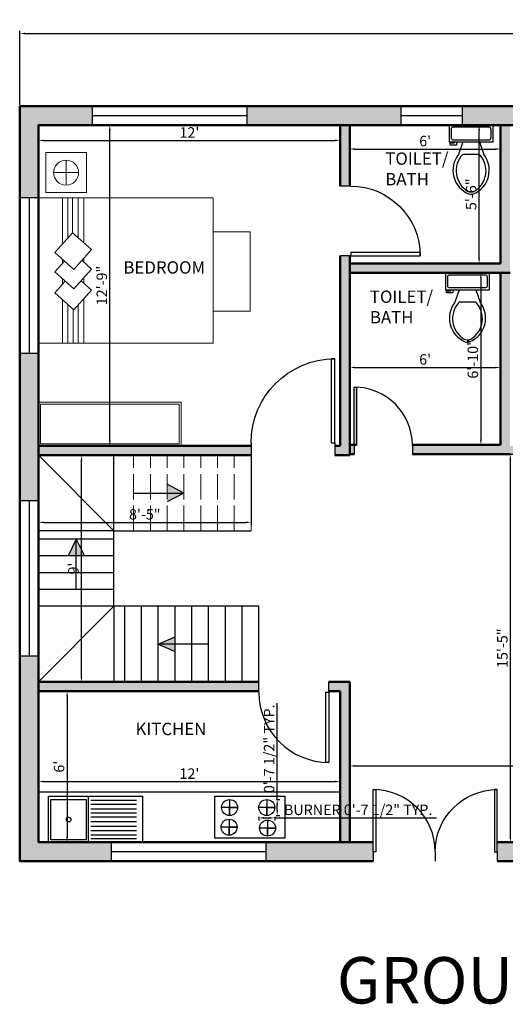
# Model space of a CAD drawing. Units: inches. Extents: x 1882 to 2467, y 1298 to 1767.
# Tile 1 of 2: x 1882 to 2114, y 1298 to 1767. Entities that reach past the tile are written whole.
import ezdxf

# ---------------------------------------------------------------- set-up
doc = ezdxf.new("R2010")
doc.units = ezdxf.units.IN
doc.linetypes.add('ACAD_ISO02W100', pattern=[15, 12, -3])
for name, color, linetype, lineweight in [('A-ANNO-DIMS', 2, 'Continuous', 18), ('A-ANNO-TEXT', 7, 'Continuous', 35), ('A-AREA-IDEN', 7, 'Continuous', 25), ('A-FLOR-FIXT', 9, 'Continuous', 25), ('A-FLOR-STRS', 7, 'Continuous', 25), ('A-FLOR-STRS-OVHD', 7, 'ACAD_ISO02W100', 18), ('A-FLOR-STRS-PATT', 7, 'Continuous', 13), ('A-FURN', 8, 'Continuous', 18), ('A-WALL-PATT', 160, 'Continuous', 13), ('DOOR', 140, 'Continuous', 25), ('KIT', 10, 'Continuous', 25), ('WALL', 160, 'Continuous', 50), ('WIND', 52, 'Continuous', 25)]:
    doc.layers.add(name, color=color, linetype=linetype, lineweight=lineweight)
doc.styles.get("Standard").update_dxf_attribs({"font": 'arial.ttf'})
doc.dimstyles.new('ISO-25', dxfattribs={"dimtxt": 5, "dimasz": 2.5, "dimexe": 1.25, "dimexo": 0.625, "dimtad": 1, "dimdec": 0, "dimlunit": 4, "dimtxsty": 'Standard', "dimcen": 2.5, "dimadec": 0, "dimazin": 0, "dimtfac": 1, "dimtdec": 0, "dimtmove": 0, "dimatfit": 3, "dimfxl": 1, "dimarcsym": 0})

# ---------------------------------------------------------------- blocks, each defined once
blk = doc.blocks.new('*U2')
for p, q in [((0, 0), (0, -6)), ((40, 0), (40, -6))]:
    blk.add_line(p, q)
blk.add_lwpolyline([(0, 0), (0, 40), (1.75, 40), (1.75, 0)], close=True)
blk.add_arc((0, 0), 40, 0, 90)
blk = doc.blocks.new('*U4')
for p, q in [((9.5, -6), (9.5, -2)), ((-10, -8.5), (-8, -8.5)), ((-10, -9.5), (-10, -8.5)), ((-8, -8.5), (-8, -8)), ((-7, -8), (-7, -9.5)), ((-4, -8), (-6, -14)), ((4, -8), (6, -14)), ((-7, -9.5), (-10, -9.5)), ((4, -14), (-4, -14))]:
    blk.add_line(p, q)
blk.add_lwpolyline([(10.5, -8), (10.5, 0), (-10.5, 0), (-10.5, -8)], close=True)
for points in [[(-9.5, -2), (-9.5, -6)], [(8.5, -1), (-8.5, -1)], [(-8.5, -7), (8.5, -7)]]:
    blk.add_lwpolyline(points)
for centre, radius, start, end in [((-8.62, -1.88), 0.884, 81.8699, 188.1301), ((8.62, -1.88), 0.884, 351.8699, 98.1301), ((-8.62, -6.12), 0.884, 171.8699, 278.1301), ((8.62, -6.12), 0.884, 261.8699, 8.1301), ((3.52, -21.58), 12.17, 141.4691, 247.9714), ((4.2, -21.82), 11.33, 136.3677, 238.9468), ((-3.52, -21.58), 12.17, 292.0284, 38.5307), ((-4.2, -21.82), 11.33, 301.053, 43.6321), ((0, -27.88), 4, 245.7318, 294.2682), ((0, -29), 4, 254.8605, 285.1395)]:
    blk.add_arc(centre, radius, start, end)
blk = doc.blocks.new('*D7')
at = {"layer": 'A-ANNO-DIMS', "color": 0, "lineweight": -2, "transparency": 16777216}
for p, q in [((1891.22, 1716.45), (1891.22, 1708.51)), ((2035.22, 1716.45), (2035.22, 1708.51)), ((1893.72, 1709.76), (2032.72, 1709.76))]:
    blk.add_line(p, q, dxfattribs=at)
at = {"layer": 'A-ANNO-DIMS', "color": 0, "lineweight": 100, "transparency": 16777216}
for points in [[(1893.72, 1710.18), (1893.72, 1709.35), (1891.22, 1709.76)], [(2032.72, 1710.18), (2032.72, 1709.35), (2035.22, 1709.76)]]:
    blk.add_solid(points, dxfattribs=at)
at = {"layer": 'Defpoints', "color": 0, "lineweight": 100, "transparency": 16777216}
for p in [(1891.22, 1717.07), (2035.22, 1717.07), (2035.22, 1709.76)]:
    blk.add_point(p, dxfattribs=at)
at = {"layer": 'A-ANNO-DIMS', "color": 0, "transparency": 16777216, "insert": (1963.22, 1712.9), "char_height": 5, "attachment_point": 5}
blk.add_mtext("12'", dxfattribs=at)
blk = doc.blocks.new('*D8')
at = {"layer": 'A-ANNO-DIMS', "color": 0, "lineweight": -2, "transparency": 16777216}
for p, q in [((1891.84, 1717.07), (1926.48, 1717.07)), ((1925.23, 1566.57), (1925.23, 1714.57)), ((1891.84, 1564.07), (1926.48, 1564.07))]:
    blk.add_line(p, q, dxfattribs=at)
at = {"layer": 'A-ANNO-DIMS', "color": 0, "lineweight": 100, "transparency": 16777216}
for points in [[(1924.81, 1714.57), (1925.64, 1714.57), (1925.23, 1717.07)], [(1924.81, 1566.57), (1925.64, 1566.57), (1925.23, 1564.07)]]:
    blk.add_solid(points, dxfattribs=at)
at = {"layer": 'Defpoints', "color": 0, "lineweight": 100, "transparency": 16777216}
for p in [(1891.22, 1717.07), (1925.23, 1717.07), (1891.22, 1564.07)]:
    blk.add_point(p, dxfattribs=at)
at = {"layer": 'A-ANNO-DIMS', "color": 0, "transparency": 16777216, "insert": (1922.05, 1640.57), "char_height": 5, "attachment_point": 5, "rotation": 90}
blk.add_mtext('12\'-9"', dxfattribs=at)
blk = doc.blocks.new('*D9')
at = {"layer": 'A-ANNO-DIMS', "color": 0, "lineweight": -2, "transparency": 16777216}
for p, q in [((2039.72, 1716.45), (2039.72, 1704.39)), ((2111.72, 1716.45), (2111.72, 1704.39)), ((2042.22, 1705.64), (2109.22, 1705.64))]:
    blk.add_line(p, q, dxfattribs=at)
at = {"layer": 'A-ANNO-DIMS', "color": 0, "lineweight": 100, "transparency": 16777216}
for points in [[(2042.22, 1706.05), (2042.22, 1705.22), (2039.72, 1705.64)], [(2109.22, 1706.05), (2109.22, 1705.22), (2111.72, 1705.64)]]:
    blk.add_solid(points, dxfattribs=at)
at = {"layer": 'Defpoints', "color": 0, "lineweight": 100, "transparency": 16777216}
for p in [(2039.72, 1717.07), (2111.72, 1717.07), (2111.72, 1705.64)]:
    blk.add_point(p, dxfattribs=at)
at = {"layer": 'A-ANNO-DIMS', "color": 0, "transparency": 16777216, "insert": (2075.72, 1708.81), "char_height": 5, "attachment_point": 5}
blk.add_mtext("6'", dxfattribs=at)
blk = doc.blocks.new('*D10')
at = {"layer": 'A-ANNO-DIMS', "color": 0, "lineweight": -2, "transparency": 16777216}
for p, q in [((2111.09, 1717.07), (2100.22, 1717.07)), ((2101.47, 1653.57), (2101.47, 1714.57)), ((2111.09, 1651.07), (2100.22, 1651.07))]:
    blk.add_line(p, q, dxfattribs=at)
at = {"layer": 'A-ANNO-DIMS', "color": 0, "lineweight": 100, "transparency": 16777216}
for points in [[(2101.05, 1714.57), (2101.89, 1714.57), (2101.47, 1717.07)], [(2101.05, 1653.57), (2101.89, 1653.57), (2101.47, 1651.07)]]:
    blk.add_solid(points, dxfattribs=at)
at = {"layer": 'Defpoints', "color": 0, "lineweight": 100, "transparency": 16777216}
for p in [(2101.47, 1717.07), (2111.72, 1717.07), (2111.72, 1651.07)]:
    blk.add_point(p, dxfattribs=at)
at = {"layer": 'A-ANNO-DIMS', "color": 0, "transparency": 16777216, "insert": (2098.29, 1684.07), "char_height": 5, "attachment_point": 5, "rotation": 90}
blk.add_mtext('5\'-6"', dxfattribs=at)
blk = doc.blocks.new('*D17')
at = {"layer": 'A-ANNO-DIMS', "color": 0, "lineweight": -2, "transparency": 16777216}
for p, q in [((2039.72, 1375.7), (2039.72, 1412.69)), ((2042.22, 1411.44), (2336.72, 1411.44)), ((2339.22, 1375.7), (2339.22, 1412.69))]:
    blk.add_line(p, q, dxfattribs=at)
at = {"layer": 'A-ANNO-DIMS', "color": 0, "lineweight": 100, "transparency": 16777216}
for points in [[(2042.22, 1411.86), (2042.22, 1411.02), (2039.72, 1411.44)], [(2336.72, 1411.86), (2336.72, 1411.02), (2339.22, 1411.44)]]:
    blk.add_solid(points, dxfattribs=at)
at = {"layer": 'Defpoints', "color": 0, "lineweight": 100, "transparency": 16777216}
for p in [(2339.22, 1411.44), (2039.72, 1375.07), (2339.22, 1375.07)]:
    blk.add_point(p, dxfattribs=at)
at = {"layer": 'A-ANNO-DIMS', "color": 0, "transparency": 16777216, "insert": (2189.47, 1414.62), "char_height": 5, "attachment_point": 5}
blk.add_mtext("25'", dxfattribs=at)
blk = doc.blocks.new('*D18')
at = {"layer": 'A-ANNO-DIMS', "color": 0, "lineweight": -2, "transparency": 16777216}
for p, q in [((1891.22, 1375.7), (1891.22, 1405.24)), ((2035.22, 1375.7), (2035.22, 1405.24)), ((1893.72, 1403.99), (2032.72, 1403.99))]:
    blk.add_line(p, q, dxfattribs=at)
at = {"layer": 'A-ANNO-DIMS', "color": 0, "lineweight": 100, "transparency": 16777216}
for points in [[(1893.72, 1404.4), (1893.72, 1403.57), (1891.22, 1403.99)], [(2032.72, 1404.4), (2032.72, 1403.57), (2035.22, 1403.99)]]:
    blk.add_solid(points, dxfattribs=at)
at = {"layer": 'Defpoints', "color": 0, "lineweight": 100, "transparency": 16777216}
for p in [(2035.22, 1403.99), (1891.22, 1375.07), (2035.22, 1375.07)]:
    blk.add_point(p, dxfattribs=at)
at = {"layer": 'A-ANNO-DIMS', "color": 0, "transparency": 16777216, "insert": (1963.22, 1407.12), "char_height": 5, "attachment_point": 5}
blk.add_mtext("12'", dxfattribs=at)
blk = doc.blocks.new('*D19')
at = {"layer": 'A-ANNO-DIMS', "color": 0, "lineweight": -2, "transparency": 16777216}
for p, q in [((1891.84, 1447.07), (1906.1, 1447.07)), ((1904.85, 1444.57), (1904.85, 1377.57)), ((1891.84, 1375.07), (1906.1, 1375.07))]:
    blk.add_line(p, q, dxfattribs=at)
at = {"layer": 'A-ANNO-DIMS', "color": 0, "lineweight": 100, "transparency": 16777216}
for points in [[(1904.43, 1444.57), (1905.27, 1444.57), (1904.85, 1447.07)], [(1904.43, 1377.57), (1905.27, 1377.57), (1904.85, 1375.07)]]:
    blk.add_solid(points, dxfattribs=at)
at = {"layer": 'Defpoints', "color": 0, "lineweight": 100, "transparency": 16777216}
for p in [(1891.22, 1447.07), (1891.22, 1375.07), (1904.85, 1375.07)]:
    blk.add_point(p, dxfattribs=at)
at = {"layer": 'A-ANNO-DIMS', "color": 0, "transparency": 16777216, "insert": (1901.67, 1411.07), "char_height": 5, "attachment_point": 5, "rotation": 90}
blk.add_mtext("6'", dxfattribs=at)
blk = doc.blocks.new('*D20')
at = {"layer": 'A-ANNO-DIMS', "color": 0, "lineweight": -2, "transparency": 16777216}
for p, q in [((1891.84, 1559.57), (1912.93, 1559.57)), ((1911.68, 1454.07), (1911.68, 1557.07)), ((1891.84, 1451.57), (1912.93, 1451.57))]:
    blk.add_line(p, q, dxfattribs=at)
at = {"layer": 'A-ANNO-DIMS', "color": 0, "lineweight": 100, "transparency": 16777216}
for points in [[(1911.27, 1557.07), (1912.1, 1557.07), (1911.68, 1559.57)], [(1911.27, 1454.07), (1912.1, 1454.07), (1911.68, 1451.57)]]:
    blk.add_solid(points, dxfattribs=at)
at = {"layer": 'Defpoints', "color": 0, "lineweight": 100, "transparency": 16777216}
for p in [(1891.22, 1559.57), (1911.68, 1559.57), (1891.22, 1451.57)]:
    blk.add_point(p, dxfattribs=at)
at = {"layer": 'A-ANNO-DIMS', "color": 0, "transparency": 16777216, "insert": (1908.51, 1505.57), "char_height": 5, "attachment_point": 5, "rotation": 90}
blk.add_mtext("9'", dxfattribs=at)
blk = doc.blocks.new('*D21')
at = {"layer": 'A-ANNO-DIMS', "color": 0, "lineweight": -2, "transparency": 16777216}
for p, q in [((1891.22, 1558.95), (1891.22, 1526.34)), ((1992.61, 1558.95), (1992.61, 1526.34)), ((1893.72, 1527.59), (1990.11, 1527.59))]:
    blk.add_line(p, q, dxfattribs=at)
at = {"layer": 'A-ANNO-DIMS', "color": 0, "lineweight": 100, "transparency": 16777216}
for points in [[(1893.72, 1528.01), (1893.72, 1527.17), (1891.22, 1527.59)], [(1990.11, 1528.01), (1990.11, 1527.17), (1992.61, 1527.59)]]:
    blk.add_solid(points, dxfattribs=at)
at = {"layer": 'Defpoints', "color": 0, "lineweight": 100, "transparency": 16777216}
for p in [(1891.22, 1559.57), (1992.61, 1559.57), (1992.61, 1527.59)]:
    blk.add_point(p, dxfattribs=at)
at = {"layer": 'A-ANNO-DIMS', "color": 0, "transparency": 16777216, "insert": (1941.92, 1530.77), "char_height": 5, "attachment_point": 5}
blk.add_mtext('8\'-5"', dxfattribs=at)
blk = doc.blocks.new('*D22')
at = {"layer": 'A-ANNO-DIMS', "color": 0, "lineweight": -2, "transparency": 16777216}
for p, q in [((2039.72, 1645.95), (2039.72, 1600.23)), ((2111.72, 1645.95), (2111.72, 1600.23)), ((2042.22, 1601.48), (2109.22, 1601.48))]:
    blk.add_line(p, q, dxfattribs=at)
at = {"layer": 'A-ANNO-DIMS', "color": 0, "lineweight": 100, "transparency": 16777216}
for points in [[(2042.22, 1601.89), (2042.22, 1601.06), (2039.72, 1601.48)], [(2109.22, 1601.89), (2109.22, 1601.06), (2111.72, 1601.48)]]:
    blk.add_solid(points, dxfattribs=at)
at = {"layer": 'Defpoints', "color": 0, "lineweight": 100, "transparency": 16777216}
for p in [(2039.72, 1646.57), (2111.72, 1646.57), (2111.72, 1601.48)]:
    blk.add_point(p, dxfattribs=at)
at = {"layer": 'A-ANNO-DIMS', "color": 0, "transparency": 16777216, "insert": (2075.72, 1604.65), "char_height": 5, "attachment_point": 5}
blk.add_mtext("6'", dxfattribs=at)
blk = doc.blocks.new('*D23')
at = {"layer": 'A-ANNO-DIMS', "color": 0, "lineweight": -2, "transparency": 16777216}
for p, q in [((2111.09, 1646.57), (2101.04, 1646.57)), ((2102.29, 1644.07), (2102.29, 1567.07)), ((2111.09, 1564.57), (2101.04, 1564.57))]:
    blk.add_line(p, q, dxfattribs=at)
at = {"layer": 'A-ANNO-DIMS', "color": 0, "lineweight": 100, "transparency": 16777216}
for points in [[(2101.87, 1644.07), (2102.7, 1644.07), (2102.29, 1646.57)], [(2101.87, 1567.07), (2102.7, 1567.07), (2102.29, 1564.57)]]:
    blk.add_solid(points, dxfattribs=at)
at = {"layer": 'Defpoints', "color": 0, "lineweight": 100, "transparency": 16777216}
for p in [(2111.72, 1646.57), (2102.29, 1564.57), (2111.72, 1564.57)]:
    blk.add_point(p, dxfattribs=at)
at = {"layer": 'A-ANNO-DIMS', "color": 0, "transparency": 16777216, "insert": (2099.11, 1605.57), "char_height": 5, "attachment_point": 5, "rotation": 90}
blk.add_mtext('6\'-10"', dxfattribs=at)
blk = doc.blocks.new('*D24')
at = {"layer": 'A-ANNO-DIMS', "color": 0, "lineweight": -2, "transparency": 16777216}
for p, q in [((2110.74, 1560.07), (2117.62, 1560.07)), ((2116.37, 1377.57), (2116.37, 1557.57)), ((2110.74, 1375.07), (2117.62, 1375.07))]:
    blk.add_line(p, q, dxfattribs=at)
at = {"layer": 'A-ANNO-DIMS', "color": 0, "lineweight": 100, "transparency": 16777216}
for points in [[(2115.96, 1557.57), (2116.79, 1557.57), (2116.37, 1560.07)], [(2115.96, 1377.57), (2116.79, 1377.57), (2116.37, 1375.07)]]:
    blk.add_solid(points, dxfattribs=at)
at = {"layer": 'Defpoints', "color": 0, "lineweight": 100, "transparency": 16777216}
for p in [(2110.11, 1560.07), (2116.37, 1560.07), (2110.11, 1375.07)]:
    blk.add_point(p, dxfattribs=at)
at = {"layer": 'A-ANNO-DIMS', "color": 0, "transparency": 16777216, "insert": (2113.2, 1467.57), "char_height": 5, "attachment_point": 5, "rotation": 90}
blk.add_mtext('15\'-5"', dxfattribs=at)
blk = doc.blocks.new('*D26')
at = {"layer": 'A-ANNO-DIMS', "color": 0, "lineweight": -2, "transparency": 16777216}
for p, q in [((1882.22, 1726.7), (1882.22, 1762.02)), ((2422.22, 1726.7), (2422.22, 1762.02)), ((1884.72, 1760.77), (2419.72, 1760.77))]:
    blk.add_line(p, q, dxfattribs=at)
at = {"layer": 'A-ANNO-DIMS', "color": 0, "lineweight": 100, "transparency": 16777216}
for points in [[(1884.72, 1761.18), (1884.72, 1760.35), (1882.22, 1760.77)], [(2419.72, 1761.18), (2419.72, 1760.35), (2422.22, 1760.77)]]:
    blk.add_solid(points, dxfattribs=at)
at = {"layer": 'Defpoints', "color": 0, "lineweight": 100, "transparency": 16777216}
for p in [(2422.22, 1760.77), (1882.22, 1726.07), (2422.22, 1726.07)]:
    blk.add_point(p, dxfattribs=at)
at = {"layer": 'A-ANNO-DIMS', "color": 0, "transparency": 16777216, "insert": (2152.22, 1763.93), "char_height": 5, "attachment_point": 5}
blk.add_mtext("45'", dxfattribs=at)
blk = doc.blocks.new('WIN-74IN')
blk.add_line((0, 4.5), (74.03, 4.5))
blk.add_lwpolyline([(0, 0), (74.03, 0), (74.03, 9), (0, 9)], close=True)
blk = doc.blocks.new('BED-DOUBLE')
for p, q in [((11.49, 47.34), (11.49, 69.21)), ((14, 50.17), (14, 69.21)), ((16.17, 52.63), (16.17, 69.21)), ((18.98, 50.15), (18.98, 69.21)), ((21.58, 47.84), (21.58, 69.21)), ((11.49, 38.12), (11.49, 39.83)), ((21.58, 38.62), (21.58, 40.3)), ((11.49, 28.1), (11.49, 30.61)), ((21.58, 28.61), (21.58, 31.07)), ((11.49, 0), (11.49, 20.59)), ((21.58, 0), (21.58, 21.06)), ((14, 0), (14, 18.37)), ((16.55, 0), (16.55, 16.12)), ((18.98, 0), (18.98, 18.12))]:
    blk.add_line(p, q)
for points in [[(0, 69.21), (83.41, 69.21), (83.41, 0), (0, 0)], [(7.76, 43.13), (16.17, 52.63), (25.33, 44.53), (16.92, 35.02)], [(83.41, 15.22), (100.98, 15.22), (100.98, 53.07), (83.41, 53.07)]]:
    blk.add_lwpolyline(points, close=True)
for points in [[(20.75, 39.36), (25.33, 35.3), (16.92, 25.8), (7.76, 33.9), (12.34, 39.08)], [(20.36, 29.69), (25.33, 25.29), (16.92, 15.79), (7.76, 23.89), (12.73, 29.51)]]:
    blk.add_lwpolyline(points)
blk = doc.blocks.new('NIGHTSTAND-LAMP')
for p, q in [((9.73, 9.55), (9.73, 15.52)), ((9.73, 15.52), (9.73, 3.59)), ((15.7, 9.55), (3.77, 9.55)), ((9.73, 3.59), (9.73, 9.55)), ((9.73, 9.55), (15.7, 9.55))]:
    blk.add_line(p, q)
blk.add_lwpolyline([(0, 0), (19.47, 0), (19.47, 19.1), (0, 19.1)], close=True)
blk.add_circle((9.73, 9.55), 5.97)
blk = doc.blocks.new('COOKTOP-BURNER')
for p, q in [((3.82, 7.64), (3.82, 0)), ((7.64, 3.82), (0, 3.82)), ((3.82, 0), (3.82, 3.82)), ((3.82, 3.82), (7.64, 3.82))]:
    blk.add_line(p, q)
blk.add_circle((3.82, 3.82), 3.82)
blk = doc.blocks.new('*D35')
at = {"layer": 'A-ANNO-DIMS', "color": 0, "lineweight": -2, "transparency": 16777216}
for p, q in [((1996.32, 1387.16), (1996.32, 1385.39)), ((1998.82, 1386.64), (2001.46, 1386.64)), ((2003.96, 1387.16), (2003.96, 1385.39)), ((2003.96, 1386.64), (2081.06, 1386.64))]:
    blk.add_line(p, q, dxfattribs=at)
at = {"layer": 'A-ANNO-DIMS', "color": 0, "lineweight": 100, "transparency": 16777216}
for points in [[(1998.82, 1387.05), (1998.82, 1386.22), (1996.32, 1386.64)], [(2001.46, 1387.05), (2001.46, 1386.22), (2003.96, 1386.64)]]:
    blk.add_solid(points, dxfattribs=at)
at = {"layer": 'Defpoints', "color": 0, "lineweight": 100, "transparency": 16777216}
for p in [(1996.32, 1387.78), (2003.96, 1387.78), (2003.96, 1386.64)]:
    blk.add_point(p, dxfattribs=at)
at = {"layer": 'A-ANNO-DIMS', "color": 0, "transparency": 16777216, "insert": (2043.76, 1389.85), "char_height": 5, "attachment_point": 5}
blk.add_mtext('BURNER 0\'-7 1/2" TYP.', dxfattribs=at)
blk = doc.blocks.new('*D36')
at = {"layer": 'A-ANNO-DIMS', "color": 0, "lineweight": -2, "transparency": 16777216}
for p, q in [((2005.11, 1395.42), (2005.11, 1441.3)), ((2004.59, 1395.42), (2006.36, 1395.42)), ((2005.11, 1390.28), (2005.11, 1392.92)), ((2004.59, 1387.78), (2006.36, 1387.78))]:
    blk.add_line(p, q, dxfattribs=at)
at = {"layer": 'A-ANNO-DIMS', "color": 0, "lineweight": 100, "transparency": 16777216}
for points in [[(2004.69, 1392.92), (2005.53, 1392.92), (2005.11, 1395.42)], [(2004.69, 1390.28), (2005.53, 1390.28), (2005.11, 1387.78)]]:
    blk.add_solid(points, dxfattribs=at)
at = {"layer": 'Defpoints', "color": 0, "lineweight": 100, "transparency": 16777216}
for p in [(2003.96, 1395.42), (2005.11, 1395.42), (2003.96, 1387.78)]:
    blk.add_point(p, dxfattribs=at)
at = {"layer": 'A-ANNO-DIMS', "color": 0, "transparency": 16777216, "insert": (2001.9, 1419.61), "char_height": 5, "attachment_point": 5, "rotation": 90}
blk.add_mtext('0\'-7 1/2" TYP.', dxfattribs=at)

msp = doc.modelspace()

# ---------------------------------------------------------------- hatches: boundary and pattern name
at = {"layer": 'A-FLOR-STRS-PATT'}
h = msp.add_hatch(color=256, dxfattribs=at)
h.dxf.hatch_style = 1
h.paths.add_polyline_path([(1960.61, 1541.57), (1952.61, 1541.57), (1952.61, 1537.32)])
h.paths.add_polyline_path([(1952.61, 1545.83), (1952.61, 1541.57), (1960.61, 1541.57)])
h.paths.add_polyline_path([(1909.22, 1519.57), (1905.31, 1511.57), (1909.22, 1511.57)])
h.paths.add_polyline_path([(1909.22, 1519.57), (1909.22, 1511.57), (1913.12, 1511.57)])
h.paths.add_polyline_path([(1956.36, 1473.06), (1948.36, 1469.57), (1956.36, 1469.57)])
h.paths.add_polyline_path([(1956.36, 1469.57), (1948.36, 1469.57), (1956.36, 1466.09)])
at = {"layer": 'A-WALL-PATT'}
h = msp.add_hatch(color=256, dxfattribs=at)
h.dxf.hatch_style = 1
h.paths.add_polyline_path([(1916.77, 1726.07), (1882.22, 1726.07), (1882.22, 1682.34), (1891.22, 1682.34), (1891.22, 1717.07), (1916.77, 1717.07)])
h.paths.add_polyline_path([(2064.04, 1726.07), (1990.8, 1726.07), (1990.8, 1717.07), (2035.22, 1717.07), (2064.04, 1717.07)])
h.paths.add_polyline_path([(2149.78, 1726.07), (2093.48, 1726.07), (2093.48, 1717.07), (2108.14, 1717.07), (2111.72, 1717.07), (2149.78, 1717.07)])
h.paths.add_polyline_path([(2116.22, 1717.07), (2111.72, 1717.07), (2111.72, 1651.07), (2039.72, 1651.07), (2039.72, 1646.57), (2116.22, 1646.57)])
h.paths.add_polyline_path([(2039.72, 1717.07), (2035.22, 1717.07), (2035.22, 1687.94), (2039.72, 1687.94)])
h.paths.add_polyline_path([(1891.22, 1608.31), (1882.22, 1608.31), (1882.22, 1537.91), (1891.22, 1537.91)])
h.paths.add_polyline_path([(2039.72, 1654.79), (2035.22, 1654.79), (2035.22, 1564.07), (2032.61, 1564.07), (2032.61, 1559.57), (2039.72, 1559.57)])
h.paths.add_polyline_path([(2043.01, 1592.08), (2043.01, 1564.25), (2041.79, 1564.25), (2041.79, 1592.11), (2043.01, 1592.11), (2043.01, 1592.08, -0.398105), (2069.65, 1564.57), (2111.72, 1564.57), (2111.72, 1646.57), (2116.22, 1646.57), (2116.22, 1560.07), (2069.65, 1560.07), (2069.65, 1564.25, 0.401453)])
h.paths.add_polyline_path([(2120.13, 1564.07), (2116.22, 1564.07), (2116.22, 1560.07), (2120.13, 1560.07)])
h.paths.add_polyline_path([(2271.23, 1564.07), (2264.72, 1564.07), (2264.72, 1560.07), (2271.23, 1560.07)])
h.paths.add_polyline_path([(2303.68, 1726.07), (2223.81, 1726.07), (2223.81, 1717.07), (2260.22, 1717.07), (2303.68, 1717.07)])
h.paths.add_polyline_path([(2422.22, 1726.07), (2377.71, 1726.07), (2377.71, 1717.07), (2413.22, 1717.07), (2413.22, 1671.81), (2422.22, 1671.81)])
h = msp.add_hatch(color=256, dxfattribs=at)
h.dxf.hatch_style = 1
h.paths.add_polyline_path([(2413.22, 1564.07), (2311.23, 1564.07), (2311.23, 1560.07), (2413.22, 1560.07)])
h.paths.add_polyline_path([(2422.22, 1597.77), (2413.22, 1597.77), (2413.22, 1546.07), (2422.22, 1546.07)])
h.paths.add_polyline_path([(2422.22, 1472.04), (2413.22, 1472.04), (2413.22, 1375.07), (2407.41, 1375.07), (2407.41, 1366.07), (2422.22, 1366.07)])
h.paths.add_polyline_path([(2343.72, 1459.07), (2358.61, 1459.07), (2358.61, 1463.57), (2339.22, 1463.57), (2339.22, 1375.07), (2343.72, 1375.07)])
h.paths.add_polyline_path([(2357.52, 1375.07), (2235.04, 1375.07), (2235.04, 1366.07), (2357.52, 1366.07)])
h.paths.add_polyline_path([(2413.22, 1463.57), (2398.81, 1463.57), (2398.81, 1459.07), (2413.22, 1459.07)])
h.paths.add_polyline_path([(2161.01, 1375.07), (2110.11, 1375.07), (2110.11, 1370.52), (2110.11, 1366.07), (2161.01, 1366.07)])
h.paths.add_polyline_path([(2050.88, 1375.07), (1999.86, 1375.07), (1999.86, 1366.07), (2050.88, 1366.07), (2050.88, 1370.52)])
h.paths.add_polyline_path([(2039.72, 1451.57), (2029.82, 1451.57), (2029.82, 1447.07), (2035.22, 1447.07), (2035.22, 1375.07), (2039.72, 1375.07)])
h.paths.add_polyline_path([(1891.22, 1399.07), (1891.22, 1463.87), (1882.22, 1463.87), (1882.22, 1366.07), (1925.83, 1366.07), (1925.83, 1375.07), (1891.22, 1375.07)])
h = msp.add_hatch(color=256, dxfattribs=at)
h.dxf.hatch_style = 1
h.paths.add_polyline_path([(2041.79, 1564.25), (2041.79, 1564.57), (2039.72, 1564.57), (2039.72, 1560.07), (2041.79, 1560.07)])
h.paths.add_polyline_path([(1992.61, 1564.07), (1891.22, 1564.07), (1891.22, 1559.57), (1992.61, 1559.57)])
h.paths.add_polyline_path([(1996.36, 1451.57), (1891.22, 1451.57), (1891.22, 1447.07), (1996.36, 1447.07)])

# ---------------------------------------------------------------- linework, layer by layer
at = {"layer": 'A-FLOR-STRS'}
for p, q in [((1927.22, 1523.57), (1891.22, 1559.57)), ((1927.22, 1523.57), (1927.22, 1559.57)), ((1960.61, 1541.57), (1952.61, 1545.83)), ((1936.61, 1541.57), (1960.61, 1541.57)), ((1960.61, 1541.57), (1952.61, 1537.32)), ((1927.22, 1523.57), (1891.22, 1523.57)), ((1927.22, 1487.57), (1927.22, 1523.57)), ((1927.22, 1523.57), (1992.61, 1523.57)), ((1927.22, 1519.57), (1891.22, 1519.57)), ((1909.22, 1519.57), (1905.31, 1511.57)), ((1909.22, 1495.57), (1909.22, 1519.57)), ((1909.22, 1519.57), (1913.12, 1511.57)), ((1927.22, 1511.57), (1891.22, 1511.57)), ((1927.22, 1503.57), (1891.22, 1503.57)), ((1927.22, 1495.57), (1891.22, 1495.57)), ((1927.22, 1487.57), (1891.22, 1487.57)), ((1927.22, 1487.57), (1891.22, 1451.57)), ((1996.36, 1487.57), (1927.22, 1487.57)), ((1927.22, 1487.57), (1927.22, 1451.57)), ((1932.36, 1451.57), (1932.36, 1487.57)), ((1940.36, 1451.57), (1940.36, 1487.57)), ((1948.36, 1451.57), (1948.36, 1487.57)), ((1956.36, 1451.57), (1956.36, 1487.57)), ((1964.36, 1451.57), (1964.36, 1487.57)), ((1972.36, 1451.57), (1972.36, 1487.57)), ((1980.36, 1451.57), (1980.36, 1487.57)), ((1988.36, 1451.57), (1988.36, 1487.57)), ((1996.36, 1451.57), (1996.36, 1487.57)), ((1948.36, 1469.57), (1956.36, 1473.06)), ((1972.36, 1469.57), (1948.36, 1469.57)), ((1948.36, 1469.57), (1956.36, 1466.09))]:
    msp.add_line(p, q, dxfattribs=at)
at = {"layer": 'A-FLOR-STRS-OVHD'}
for p, q in [((1936.61, 1523.57), (1936.61, 1559.57)), ((1944.61, 1523.57), (1944.61, 1559.57)), ((1952.61, 1523.57), (1952.61, 1559.57)), ((1960.61, 1523.57), (1960.61, 1559.57)), ((1968.61, 1523.57), (1968.61, 1559.57)), ((1976.61, 1523.57), (1976.61, 1559.57)), ((1984.61, 1523.57), (1984.61, 1559.57)), ((1992.61, 1523.57), (1992.61, 1559.57)), ((1992.61, 1523.57), (1992.61, 1559.57)), ((1992.61, 1559.57), (1992.61, 1523.57)), ((1972.36, 1469.57), (1948.36, 1469.57))]:
    msp.add_line(p, q, dxfattribs=at)
at = {"layer": 'A-FURN'}
for points in [[(1891.22, 1564.07), (1959.28, 1564.07), (1959.28, 1584.96), (1891.22, 1584.96)], [(1892.22, 1565.07), (1958.28, 1565.07), (1958.28, 1583.96), (1892.22, 1583.96)]]:
    msp.add_lwpolyline(points, close=True, dxfattribs=at)
at = {"layer": 'KIT'}
for p, q in [((1891.22, 1375.07), (1891.22, 1399.07)), ((1891.22, 1399.07), (2035.22, 1399.07)), ((1914.83, 1396.97), (1914.83, 1375.07)), ((1916.2, 1395.1), (1937.98, 1395.1)), ((1916.2, 1393.23), (1937.98, 1393.23)), ((1916.2, 1391.05), (1937.98, 1391.05)), ((1916.2, 1389.01), (1937.98, 1389.01)), ((1916.2, 1387.09), (1937.98, 1387.09)), ((1916.2, 1385), (1937.98, 1385)), ((1916.2, 1382.78), (1937.98, 1382.78)), ((1916.2, 1380.69), (1937.98, 1380.69)), ((1916.2, 1378.64), (1937.98, 1378.64)), ((1916.2, 1376.81), (1937.98, 1376.81))]:
    msp.add_line(p, q, dxfattribs=at)
for points in [[(1896.03, 1396.97), (1940.88, 1396.97), (1940.88, 1375.07), (1896.03, 1375.07)], [(1897.16, 1395.41), (1913.97, 1395.41), (1913.97, 1376.25), (1897.16, 1376.25)], [(1975.41, 1397.04), (2008.68, 1397.04), (2008.68, 1377.05), (1975.41, 1377.05)]]:
    msp.add_lwpolyline(points, close=True, dxfattribs=at)
msp.add_circle((1905.57, 1385.83), 1.1, dxfattribs=at)
at = {"layer": 'WALL'}
for p, q in [((1882.22, 1726.07), (2422.22, 1726.07)), ((1882.22, 1366.07), (1882.22, 1726.07)), ((1891.22, 1717.07), (2035.22, 1717.07)), ((2035.22, 1717.07), (2035.22, 1687.94)), ((2039.72, 1717.07), (2039.72, 1687.94)), ((2039.72, 1717.07), (2111.72, 1717.07)), ((2111.72, 1717.07), (2111.72, 1651.07)), ((2035.22, 1654.79), (2035.22, 1564.07)), ((2039.72, 1654.79), (2039.72, 1559.57)), ((2111.72, 1651.07), (2039.72, 1651.07)), ((2116.22, 1646.57), (2039.72, 1646.57)), ((2039.72, 1646.57), (2039.72, 1564.57)), ((2111.72, 1564.57), (2111.72, 1646.57)), ((1992.61, 1564.07), (1891.22, 1564.07)), ((2035.22, 1564.07), (2032.61, 1564.07)), ((2039.72, 1564.57), (2043.01, 1564.57)), ((2069.65, 1564.57), (2111.72, 1564.57)), ((1992.61, 1559.57), (1891.22, 1559.57)), ((2039.72, 1559.57), (2032.61, 1559.57)), ((2039.72, 1560.07), (2041.79, 1560.07)), ((2069.65, 1560.07), (2116.22, 1560.07)), ((1996.36, 1451.57), (1891.22, 1451.57)), ((2039.72, 1451.57), (2029.82, 1451.57)), ((2039.72, 1375.07), (2039.72, 1451.57)), ((1996.36, 1447.07), (1891.22, 1447.07)), ((2035.22, 1447.07), (2029.82, 1447.07)), ((2035.22, 1375.07), (2035.22, 1447.07)), ((1891.22, 1375.07), (2035.22, 1375.07)), ((2039.72, 1375.07), (2050.88, 1375.07)), ((2110.11, 1375.07), (2343.72, 1375.07)), ((2050.88, 1366.07), (1882.22, 1366.07)), ((2422.22, 1366.07), (2110.11, 1366.07))]:
    msp.add_line(p, q, dxfattribs=at)
for points in [[(2050.88, 1366.07), (1882.22, 1366.07), (1882.22, 1726.07), (2422.22, 1726.07), (2422.22, 1366.07), (2110.11, 1366.07)], [(2050.88, 1375.07), (1891.22, 1375.07), (1891.22, 1717.07), (2413.22, 1717.07), (2413.22, 1375.07), (2110.11, 1375.07)]]:
    msp.add_lwpolyline(points, dxfattribs=at)
at = {"layer": 'WIND'}
msp.add_line((2064.04, 1721.57), (2093.48, 1721.57), dxfattribs=at)
msp.add_lwpolyline([(2064.04, 1717.07), (2093.48, 1717.07), (2093.48, 1726.07), (2064.04, 1726.07)], close=True, dxfattribs=at)

# ---------------------------------------------------------------- block references
at = {"layer": 'A-FLOR-FIXT'}
for p in [(2097.64, 1717.07), (2095.91, 1646.57)]:
    msp.add_blockref('*U4', p, dxfattribs=at)
at = {"layer": 'A-FURN'}
for name, p in [('NIGHTSTAND-LAMP', (1894.65, 1684.85)), ('BED-DOUBLE', (1891.22, 1613.13))]:
    msp.add_blockref(name, p, dxfattribs=at)
at = {"layer": 'DOOR'}
for p, xscale, yscale, zscale, rotation in [((2040.19, 1654.79), -0.8287132811936988, 0.8287132811936988, 0.8287132811936988, 270), ((2029.82, 1446.55), 0.8366787775190851, 0.8366787775190851, 0.8366787775190851, 180)]:
    msp.add_blockref('*U2', p, dxfattribs=dict(at, xscale=xscale, yscale=yscale, zscale=zscale, rotation=rotation))
at = {"layer": 'DOOR', "xscale": -1}
msp.add_blockref('*U2', (2032.61, 1565.57), dxfattribs=at)
at = {"layer": 'DOOR'}
for p, xscale, yscale, zscale in [((2041.79, 1564.25), 0.6964052878528265, 0.6964052878528265, 0.6964052878528265), ((2050.88, 1370.52), 0.740423804381808, 0.740423804381808, 0.740423804381808), ((2110.11, 1370.52), -0.740423804381808, 0.740423804381808, 0.740423804381808)]:
    msp.add_blockref('*U2', p, dxfattribs=dict(at, xscale=xscale, yscale=yscale, zscale=zscale))
at = {"layer": 'KIT'}
for p in [(1978.57, 1387.78), (1996.32, 1387.78), (1978.34, 1378.4), (1996.68, 1377.99)]:
    msp.add_blockref('COOKTOP-BURNER', p, dxfattribs=at)
at = {"layer": 'WIND'}
for p in [(1916.77, 1717.08), (1925.83, 1366.08)]:
    msp.add_blockref('WIN-74IN', p, dxfattribs=at)
for p, rotation in [((1882.22, 1682.34), 269.9999999999998), ((1882.22, 1537.9), 269.9999999999997)]:
    msp.add_blockref('WIN-74IN', p, dxfattribs=dict(at, rotation=rotation))

# ---------------------------------------------------------------- texts
at = {"layer": 'A-ANNO-TEXT', "insert": (2033.57, 1320.26), "char_height": 22.1185, "attachment_point": 1}
msp.add_mtext_dynamic_manual_height_columns('GROUND FLOOR', width=577.1514, gutter_width=110.59, heights=[0], dxfattribs=at)
at = {"layer": 'A-AREA-IDEN', "char_height": 5.88, "attachment_point": 1}
for s, insert in [('TOILET/\\PBATH', (2056.69, 1704.02)), ('BEDROOM', (1931.72, 1652.12)), ('TOILET/\\PBATH', (2049.35, 1638.18)), ('KITCHEN', (1937.49, 1432.01))]:
    msp.add_mtext_dynamic_manual_height_columns(s, width=153.4263, gutter_width=29.4, heights=[0], dxfattribs=dict(at, insert=insert))

# ---------------------------------------------------------------- dimensions: what is measured, and where the dimension line sits
at = {"layer": 'A-ANNO-DIMS'}
for base, p1, p2, picture, middle in [((2422.22, 1760.77), (1882.22, 1726.07), (2422.22, 1726.07), '*D26', (2152.22, 1763.93)), ((2035.22, 1709.76), (1891.22, 1717.07), (2035.22, 1717.07), '*D7', (1963.22, 1712.9)), ((2111.72, 1705.64), (2039.72, 1717.07), (2111.72, 1717.07), '*D9', (2075.72, 1708.81)), ((2111.72, 1601.48), (2039.72, 1646.57), (2111.72, 1646.57), '*D22', (2075.72, 1604.65)), ((1992.61, 1527.59), (1891.22, 1559.57), (1992.61, 1559.57), '*D21', (1941.92, 1530.77)), ((2339.21873251, 1411.44158288), (2039.71873251, 1375.07458791), (2339.21873251, 1375.07458791), '*D17', (2189.46873251, 1414.61944782)), ((2035.22, 1403.99), (1891.22, 1375.07), (2035.22, 1375.07), '*D18', (1963.22, 1407.12))]:
    dim = msp.add_linear_dim(base=base, p1=p1, p2=p2, dimstyle='ISO-25', override={"dimclrd": 0, "dimclre": 0, "dimclrt": 0}, dxfattribs=at)
    dim.commit()
    dim.dimension.update_dxf_attribs({"geometry": picture, "text_midpoint": middle})
for base, p1, p2, picture, middle in [((1925.23, 1717.07), (1891.22, 1564.07), (1891.22, 1717.07), '*D8', (1922.05, 1640.57)), ((2101.47, 1717.07), (2111.72, 1651.07), (2111.72, 1717.07), '*D10', (2098.29, 1684.07)), ((2102.29, 1564.57), (2111.72, 1646.57), (2111.72, 1564.57), '*D23', (2099.11, 1605.57)), ((1911.68, 1559.57), (1891.22, 1451.57), (1891.22, 1559.57), '*D20', (1908.51, 1505.57)), ((2116.37, 1560.07), (2110.11, 1375.07), (2110.11, 1560.07), '*D24', (2113.2, 1467.57)), ((1904.85, 1375.07), (1891.22, 1447.07), (1891.22, 1375.07), '*D19', (1901.67, 1411.07))]:
    dim = msp.add_linear_dim(base=base, p1=p1, p2=p2, angle=90, dimstyle='ISO-25', override={"dimclrd": 0, "dimclre": 0, "dimclrt": 0}, dxfattribs=at)
    dim.commit()
    dim.dimension.update_dxf_attribs({"geometry": picture, "text_midpoint": middle})
dim = msp.add_linear_dim(base=(2005.11, 1395.42), p1=(2003.96, 1387.78), p2=(2003.96, 1395.42), angle=90, text='<> TYP.', dimstyle='ISO-25', override={"dimdec": 1, "dimlfac": 1, "dimrnd": 0, "dimzin": 1, "dimdsep": 46, "dimlunit": 4, "dimfrac": 2}, dxfattribs=at)
dim.commit()
dim.dimension.update_dxf_attribs({"geometry": '*D36', "text_midpoint": (2001.9, 1419.61)})
dim = msp.add_linear_dim(base=(2003.96, 1386.64), p1=(1996.32, 1387.78), p2=(2003.96, 1387.78), text='BURNER <> TYP.', dimstyle='ISO-25', override={"dimdec": 1, "dimlfac": 1, "dimrnd": 0, "dimzin": 1, "dimdsep": 46, "dimlunit": 4, "dimfrac": 2}, dxfattribs=at)
dim.commit()
dim.dimension.update_dxf_attribs({"geometry": '*D35', "text_midpoint": (2043.76, 1389.85)})

doc.saveas('drawing.dxf')
